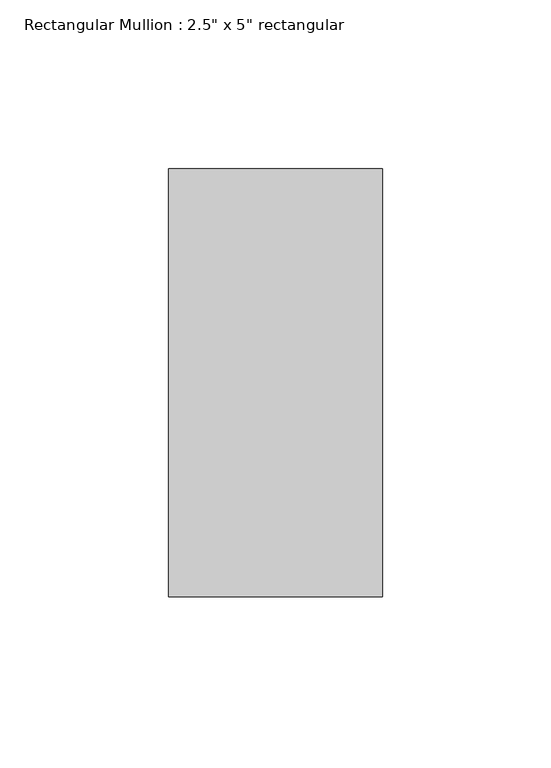
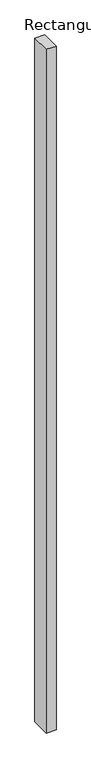
"""IFC4 building model written with IfcOpenShell, lengths in millimetres: member geometry."""

from ifc_helpers import new_model, si_unit, frame, origin, place, context, project, spatial, polyline, outline, extrude, source, transform, mapped, element, save


def member_35409717(model_context):
    return source(origin(), model_context, "Body", "SweptSolid", [
        extrude(outline(polyline([(0.0, 63.5), (0.0, -63.5), (-63.5, -63.5), (-63.5, 63.5), (0.0, 63.5)])), frame((0.0, 0.0, -4686.3), z_axis=(0.0, 0.0, 1.0), x_axis=(1.0, 0.0, 0.0)), (0.0, 0.0, 1.0), 4686.3),
    ])


if __name__ == "__main__":
    model = new_model("IFC4")
    model_context = context("Model", 3, world=origin())
    ifc_project = project(units=[si_unit("LENGTHUNIT", "METRE", prefix="MILLI")], contexts=[model_context])
    site = spatial("IfcSite", under=ifc_project)
    building = spatial("IfcBuilding", under=site)
    placement = place(None, origin())
    member_shape = member_35409717(model_context)
    element("IfcMember", 1, ObjectType="Rectangular Mullion : 2.5\" x 5\" rectangular", at=placement, inside=building, context=model_context, shape_type="MappedRepresentation", body=[
        mapped(member_shape, transform((0.0, 0.0, 0.0), x_axis=(1.0, 0.0, 0.0), y_axis=(0.0, 1.0, 0.0), z_axis=(0.0, 0.0, 1.0))),
    ])
    save(model, "model.ifc")

# Revit data of these elements
# Type "Rectangular Mullion : 2.5\" x 5\" rectangular"
#   built-in parameter 1007304 = 0.416667 (stored number, unit not read)
#   built-in parameter 1007301 = 0.104167 (stored number, unit not read)
#   built-in parameter 1007300 = 0.104167 (stored number, unit not read)
# Element 1 (IfcMember, "Rectangular Mullion : 2.5\" x 5\" rectangular")
#   Materials on its faces: "Aluminum"
# Materials
#   "Aluminum": class "Metal", colour RGB 247 247 247, transparency 0, Description = "Aluminum 6061", Cost = 0
